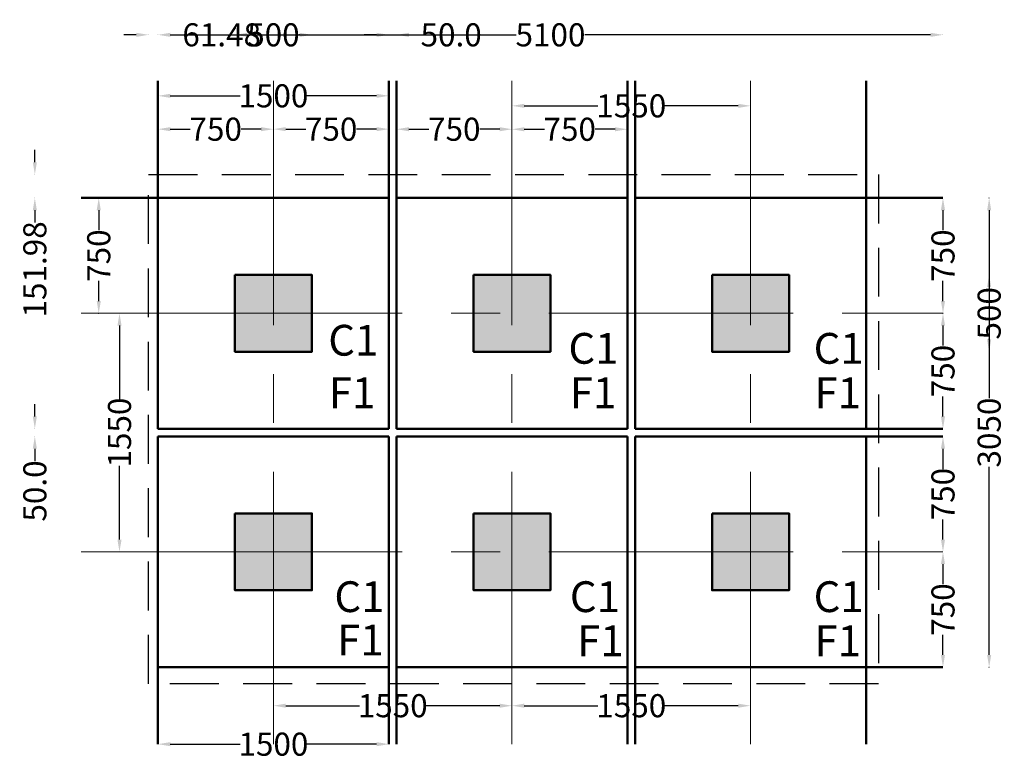
# Model space of a CAD drawing. Units: millimetres. Extents: x -19888 to 14444, y 67066 to 90098.
# Tile 4 of 7: x -19888 to -13491, y 82312 to 87118. Entities that reach past the tile are written whole.
import ezdxf

# ---------------------------------------------------------------- set-up
doc = ezdxf.new("R2010")
doc.units = ezdxf.units.MM
doc.header["$LTSCALE"] = 50
doc.header["$MEASUREMENT"] = 0
doc.linetypes.add('CENTER', pattern=[50.8, 31.75, -6.35, 6.35, -6.35])
doc.linetypes.add('HIDDEN', pattern=[9.525, 6.35, -3.175])
for name, color, linetype, lineweight in [('S-ANNO-DIMS', 2, 'Continuous', 18), ('S-ANNO-TEXT', 7, 'Continuous', 25), ('S-COLS', 4, 'Continuous', 50), ('S-FNDN', 1, 'Continuous', 50), ('S-FNDN-HIDN', 1, 'HIDDEN', 25), ('S-GRID', 8, 'CENTER', 18), ('S-PATT', 8, 'Continuous', 13)]:
    doc.layers.add(name, color=color, linetype=linetype, lineweight=lineweight)
doc.styles.get("Standard").update_dxf_attribs({"font": 'arial.ttf'})
doc.dimstyles.get("Standard").update_dxf_attribs({"dimtxt": 150, "dimasz": 80, "dimexe": 0.18, "dimexo": 0.0625, "dimgap": 0.09, "dimtad": 0, "dimdec": 0, "dimzin": 0, "dimdsep": 46, "dimtxsty": 'Standard', "dimcen": 0.09, "dimadec": 0, "dimazin": 0, "dimtfac": 1, "dimtdec": 0, "dimtofl": 0, "dimtmove": 0, "dimatfit": 3, "dimfxl": 1, "dimfxlon": 1, "dimtolj": 1, "dimtzin": 0, "dimarcsym": 0})

# ---------------------------------------------------------------- blocks, each defined once
blk = doc.blocks.new('*D1')
at = {"layer": 'Defpoints', "color": 0, "transparency": 16777216}
for p in [(-18989.3, 86406.7), (-18239.3, 86406.7), (-18239.3, 86406.7)]:
    blk.add_point(p, dxfattribs=at)
at = {"layer": 'S-ANNO-DIMS', "color": 0, "lineweight": -2, "transparency": 16777216}
for p, q in [((-18989.3, 86406.7), (-18989.3, 86406.9)), ((-18909.3, 86406.7), (-18779.2, 86406.7)), ((-18319.3, 86406.7), (-18449.3, 86406.7)), ((-18239.3, 86406.7), (-18239.3, 86406.9))]:
    blk.add_line(p, q, dxfattribs=at)
at = {"layer": 'S-ANNO-DIMS', "color": 0, "transparency": 16777216}
for points in [[(-18909.3, 86420.1), (-18909.3, 86393.4), (-18989.3, 86406.7)], [(-18319.3, 86420.1), (-18319.3, 86393.4), (-18239.3, 86406.7)]]:
    blk.add_solid(points, dxfattribs=at)
at = {"layer": 'S-ANNO-DIMS', "color": 0, "transparency": 16777216, "insert": (-18614.3, 86406.7), "char_height": 150, "attachment_point": 5}
blk.add_mtext('\\A1;750', dxfattribs=at)
blk = doc.blocks.new('*D2')
at = {"layer": 'Defpoints', "color": 0, "transparency": 16777216}
for p in [(-18239.3, 86406.7), (-17489.3, 86406.9), (-17489.3, 86406.7)]:
    blk.add_point(p, dxfattribs=at)
at = {"layer": 'S-ANNO-DIMS', "color": 0, "lineweight": -2, "transparency": 16777216}
for p, q in [((-18239.3, 86406.8), (-18239.3, 86407.1)), ((-18159.3, 86406.9), (-18029.2, 86406.9)), ((-17569.3, 86406.9), (-17699.3, 86406.9)), ((-17489.3, 86406.8), (-17489.3, 86407.1))]:
    blk.add_line(p, q, dxfattribs=at)
at = {"layer": 'S-ANNO-DIMS', "color": 0, "transparency": 16777216}
for points in [[(-18159.3, 86420.3), (-18159.3, 86393.6), (-18239.3, 86406.9)], [(-17569.3, 86420.3), (-17569.3, 86393.6), (-17489.3, 86406.9)]]:
    blk.add_solid(points, dxfattribs=at)
at = {"layer": 'S-ANNO-DIMS', "color": 0, "transparency": 16777216, "insert": (-17864.3, 86406.9), "char_height": 150, "attachment_point": 5}
blk.add_mtext('\\A1;750', dxfattribs=at)
blk = doc.blocks.new('*D3')
at = {"layer": 'Defpoints', "color": 0, "transparency": 16777216}
for p in [(-18989.3, 86719.9), (-17489.3, 86719.9), (-17489.3, 86623.5)]:
    blk.add_point(p, dxfattribs=at)
at = {"layer": 'S-ANNO-DIMS', "color": 0, "lineweight": -2, "transparency": 16777216}
for p, q in [((-18989.3, 86624.5), (-18989.3, 86623.3)), ((-18909.3, 86623.5), (-18456, 86623.5)), ((-17569.3, 86623.5), (-18022.5, 86623.5)), ((-17489.3, 86624.5), (-17489.3, 86623.3))]:
    blk.add_line(p, q, dxfattribs=at)
at = {"layer": 'S-ANNO-DIMS', "color": 0, "transparency": 16777216}
for points in [[(-18909.3, 86636.8), (-18909.3, 86610.2), (-18989.3, 86623.5)], [(-17569.3, 86636.8), (-17569.3, 86610.2), (-17489.3, 86623.5)]]:
    blk.add_solid(points, dxfattribs=at)
at = {"layer": 'S-ANNO-DIMS', "color": 0, "transparency": 16777216, "insert": (-18239.3, 86623.5), "char_height": 150, "attachment_point": 5}
blk.add_mtext('\\A1;1500', dxfattribs=at)
blk = doc.blocks.new('*D4')
at = {"layer": 'Defpoints', "color": 0, "transparency": 16777216}
for p in [(-17439.3, 86406.5), (-17439.3, 86406.5), (-16689.3, 86406.5)]:
    blk.add_point(p, dxfattribs=at)
at = {"layer": 'S-ANNO-DIMS', "color": 0, "lineweight": -2, "transparency": 16777216}
for p, q in [((-17439.3, 86406.5), (-17439.3, 86406.7)), ((-17359.3, 86406.5), (-17229.2, 86406.5)), ((-16769.3, 86406.5), (-16899.3, 86406.5)), ((-16689.3, 86406.5), (-16689.3, 86406.7))]:
    blk.add_line(p, q, dxfattribs=at)
at = {"layer": 'S-ANNO-DIMS', "color": 0, "transparency": 16777216}
for points in [[(-17359.3, 86419.8), (-17359.3, 86393.2), (-17439.3, 86406.5)], [(-16769.3, 86419.8), (-16769.3, 86393.2), (-16689.3, 86406.5)]]:
    blk.add_solid(points, dxfattribs=at)
at = {"layer": 'S-ANNO-DIMS', "color": 0, "transparency": 16777216, "insert": (-17064.3, 86406.5), "char_height": 150, "attachment_point": 5}
blk.add_mtext('\\A1;750', dxfattribs=at)
blk = doc.blocks.new('*D5')
at = {"layer": 'Defpoints', "color": 0, "transparency": 16777216}
for p in [(-16689.3, 86406.5), (-15939.3, 86406.5), (-15939.3, 86406.1)]:
    blk.add_point(p, dxfattribs=at)
at = {"layer": 'S-ANNO-DIMS', "color": 0, "lineweight": -2, "transparency": 16777216}
for p, q in [((-16689.3, 86406.4), (-16689.3, 86405.9)), ((-16609.3, 86406.1), (-16479.2, 86406.1)), ((-16019.3, 86406.1), (-16149.3, 86406.1)), ((-15939.3, 86406.4), (-15939.3, 86405.9))]:
    blk.add_line(p, q, dxfattribs=at)
at = {"layer": 'S-ANNO-DIMS', "color": 0, "transparency": 16777216}
for points in [[(-16609.3, 86419.5), (-16609.3, 86392.8), (-16689.3, 86406.1)], [(-16019.3, 86419.5), (-16019.3, 86392.8), (-15939.3, 86406.1)]]:
    blk.add_solid(points, dxfattribs=at)
at = {"layer": 'S-ANNO-DIMS', "color": 0, "transparency": 16777216, "insert": (-16314.3, 86406.1), "char_height": 150, "attachment_point": 5}
blk.add_mtext('\\A1;750', dxfattribs=at)
blk = doc.blocks.new('*D6')
at = {"layer": 'Defpoints', "color": 0, "transparency": 16777216}
for p in [(-16689.3, 86719.9), (-15139.3, 86719.9), (-16689.3, 86558.4)]:
    blk.add_point(p, dxfattribs=at)
at = {"layer": 'S-ANNO-DIMS', "color": 0, "lineweight": -2, "transparency": 16777216}
for p, q in [((-16689.3, 86559.4), (-16689.3, 86558.2)), ((-16609.3, 86558.4), (-16131, 86558.4)), ((-15219.3, 86558.4), (-15697.5, 86558.4)), ((-15139.3, 86559.4), (-15139.3, 86558.2))]:
    blk.add_line(p, q, dxfattribs=at)
at = {"layer": 'S-ANNO-DIMS', "color": 0, "transparency": 16777216}
for points in [[(-16609.3, 86571.7), (-16609.3, 86545.1), (-16689.3, 86558.4)], [(-15219.3, 86571.7), (-15219.3, 86545.1), (-15139.3, 86558.4)]]:
    blk.add_solid(points, dxfattribs=at)
at = {"layer": 'S-ANNO-DIMS', "color": 0, "transparency": 16777216, "insert": (-15914.3, 86558.4), "char_height": 150, "attachment_point": 5}
blk.add_mtext('\\A1;1550', dxfattribs=at)
blk = doc.blocks.new('*D7')
at = {"layer": 'Defpoints', "color": 0, "transparency": 16777216}
for p in [(-18989.3, 82410), (-17489.3, 82410), (-17489.3, 82410)]:
    blk.add_point(p, dxfattribs=at)
at = {"layer": 'S-ANNO-DIMS', "color": 0, "lineweight": -2, "transparency": 16777216}
for p, q in [((-18989.3, 82410), (-18989.3, 82410.2)), ((-18909.3, 82410), (-18456, 82410)), ((-17569.3, 82410), (-18022.5, 82410)), ((-17489.3, 82410), (-17489.3, 82410.2))]:
    blk.add_line(p, q, dxfattribs=at)
at = {"layer": 'S-ANNO-DIMS', "color": 0, "transparency": 16777216}
for points in [[(-18909.3, 82423.4), (-18909.3, 82396.7), (-18989.3, 82410)], [(-17569.3, 82423.4), (-17569.3, 82396.7), (-17489.3, 82410)]]:
    blk.add_solid(points, dxfattribs=at)
at = {"layer": 'S-ANNO-DIMS', "color": 0, "transparency": 16777216, "insert": (-18239.3, 82410), "char_height": 150, "attachment_point": 5}
blk.add_mtext('\\A1;1500', dxfattribs=at)
blk = doc.blocks.new('*D8')
at = {"layer": 'Defpoints', "color": 0, "transparency": 16777216}
for p in [(-18239.3, 82660), (-16689.3, 82660), (-16689.3, 82660)]:
    blk.add_point(p, dxfattribs=at)
at = {"layer": 'S-ANNO-DIMS', "color": 0, "lineweight": -2, "transparency": 16777216}
for p, q in [((-18239.3, 82660), (-18239.3, 82660.2)), ((-18159.3, 82660), (-17681, 82660)), ((-16769.3, 82660), (-17247.5, 82660)), ((-16689.3, 82660), (-16689.3, 82660.2))]:
    blk.add_line(p, q, dxfattribs=at)
at = {"layer": 'S-ANNO-DIMS', "color": 0, "transparency": 16777216}
for points in [[(-18159.3, 82673.4), (-18159.3, 82646.7), (-18239.3, 82660)], [(-16769.3, 82673.4), (-16769.3, 82646.7), (-16689.3, 82660)]]:
    blk.add_solid(points, dxfattribs=at)
at = {"layer": 'S-ANNO-DIMS', "color": 0, "transparency": 16777216, "insert": (-17464.3, 82660), "char_height": 150, "attachment_point": 5}
blk.add_mtext('\\A1;1550', dxfattribs=at)
blk = doc.blocks.new('*D9')
at = {"layer": 'Defpoints', "color": 0, "transparency": 16777216}
for p in [(-16689.3, 82653.4), (-15139.3, 82660), (-15139.3, 82660)]:
    blk.add_point(p, dxfattribs=at)
at = {"layer": 'S-ANNO-DIMS', "color": 0, "lineweight": -2, "transparency": 16777216}
for p, q in [((-16689.3, 82659), (-16689.3, 82660.2)), ((-16609.3, 82660), (-16131, 82660)), ((-15219.3, 82660), (-15697.5, 82660)), ((-15139.3, 82660), (-15139.3, 82660.2))]:
    blk.add_line(p, q, dxfattribs=at)
at = {"layer": 'S-ANNO-DIMS', "color": 0, "transparency": 16777216}
for points in [[(-16609.3, 82673.4), (-16609.3, 82646.7), (-16689.3, 82660)], [(-15219.3, 82673.4), (-15219.3, 82646.7), (-15139.3, 82660)]]:
    blk.add_solid(points, dxfattribs=at)
at = {"layer": 'S-ANNO-DIMS', "color": 0, "transparency": 16777216, "insert": (-15914.3, 82660), "char_height": 150, "attachment_point": 5}
blk.add_mtext('\\A1;1550', dxfattribs=at)
blk = doc.blocks.new('*D10')
at = {"layer": 'Defpoints', "color": 0, "ltscale": 50, "transparency": 16777216}
for p in [(-19239.3, 85210), (-19239.3, 83660), (-19239.3, 83660)]:
    blk.add_point(p, dxfattribs=at)
at = {"layer": 'S-ANNO-DIMS', "color": 0, "lineweight": -2, "ltscale": 50, "transparency": 16777216}
for p, q in [((-19239.3, 85210), (-19239.4, 85210)), ((-19239.3, 85130), (-19239.3, 84651.8)), ((-19239.3, 83740), (-19239.3, 84218.3)), ((-19239.3, 83660), (-19239.4, 83660))]:
    blk.add_line(p, q, dxfattribs=at)
at = {"layer": 'S-ANNO-DIMS', "color": 0, "ltscale": 50, "transparency": 16777216}
for points in [[(-19252.6, 85130), (-19225.9, 85130), (-19239.3, 85210)], [(-19252.6, 83740), (-19225.9, 83740), (-19239.3, 83660)]]:
    blk.add_solid(points, dxfattribs=at)
at = {"layer": 'S-ANNO-DIMS', "color": 0, "ltscale": 50, "transparency": 16777216, "insert": (-19239.3, 84435), "char_height": 150, "attachment_point": 5, "rotation": 90}
blk.add_mtext('\\A1;1550', dxfattribs=at)
blk = doc.blocks.new('*D11')
at = {"layer": 'Defpoints', "color": 0, "ltscale": 50, "transparency": 16777216}
for p in [(-19489.3, 85960), (-19374.1, 85960), (-19489.3, 85210)]:
    blk.add_point(p, dxfattribs=at)
at = {"layer": 'S-ANNO-DIMS', "color": 0, "lineweight": -2, "ltscale": 50, "transparency": 16777216}
for p, q in [((-19375.1, 85960), (-19373.9, 85960)), ((-19374.1, 85880), (-19374.1, 85750)), ((-19374.1, 85290), (-19374.1, 85420.1)), ((-19375.1, 85210), (-19373.9, 85210))]:
    blk.add_line(p, q, dxfattribs=at)
at = {"layer": 'S-ANNO-DIMS', "color": 0, "ltscale": 50, "transparency": 16777216}
for points in [[(-19387.4, 85880), (-19360.7, 85880), (-19374.1, 85960)], [(-19387.4, 85290), (-19360.7, 85290), (-19374.1, 85210)]]:
    blk.add_solid(points, dxfattribs=at)
at = {"layer": 'S-ANNO-DIMS', "color": 0, "ltscale": 50, "transparency": 16777216, "insert": (-19374.1, 85585), "char_height": 150, "attachment_point": 5, "rotation": 90}
blk.add_mtext('\\A1;750', dxfattribs=at)
blk = doc.blocks.new('*D12')
at = {"layer": 'Defpoints', "color": 0, "ltscale": 50, "transparency": 16777216}
for p in [(-13889.3, 85960), (-13889.3, 85210), (-13889.3, 85210)]:
    blk.add_point(p, dxfattribs=at)
at = {"layer": 'S-ANNO-DIMS', "color": 0, "lineweight": -2, "ltscale": 50, "transparency": 16777216}
for p, q in [((-13889.3, 85960), (-13889.4, 85960)), ((-13889.3, 85880), (-13889.3, 85750)), ((-13889.3, 85290), (-13889.3, 85420.1)), ((-13889.3, 85210), (-13889.4, 85210))]:
    blk.add_line(p, q, dxfattribs=at)
at = {"layer": 'S-ANNO-DIMS', "color": 0, "ltscale": 50, "transparency": 16777216}
for points in [[(-13902.6, 85880), (-13875.9, 85880), (-13889.3, 85960)], [(-13902.6, 85290), (-13875.9, 85290), (-13889.3, 85210)]]:
    blk.add_solid(points, dxfattribs=at)
at = {"layer": 'S-ANNO-DIMS', "color": 0, "ltscale": 50, "transparency": 16777216, "insert": (-13889.3, 85585), "char_height": 150, "attachment_point": 5, "rotation": 90}
blk.add_mtext('\\A1;750', dxfattribs=at)
blk = doc.blocks.new('*D13')
at = {"layer": 'Defpoints', "color": 0, "ltscale": 50, "transparency": 16777216}
for p in [(-13889.4, 85210.1), (-13889.3, 84460), (-13889.3, 84460)]:
    blk.add_point(p, dxfattribs=at)
at = {"layer": 'S-ANNO-DIMS', "color": 0, "lineweight": -2, "ltscale": 50, "transparency": 16777216}
for p, q in [((-13889.4, 85210.1), (-13889.1, 85210.1)), ((-13889.3, 85130.1), (-13889.3, 85000)), ((-13889.3, 84540), (-13889.3, 84670.1)), ((-13889.3, 84460), (-13889.4, 84460))]:
    blk.add_line(p, q, dxfattribs=at)
at = {"layer": 'S-ANNO-DIMS', "color": 0, "ltscale": 50, "transparency": 16777216}
for points in [[(-13902.6, 85130.1), (-13875.9, 85130.1), (-13889.3, 85210.1)], [(-13902.6, 84540), (-13875.9, 84540), (-13889.3, 84460)]]:
    blk.add_solid(points, dxfattribs=at)
at = {"layer": 'S-ANNO-DIMS', "color": 0, "ltscale": 50, "transparency": 16777216, "insert": (-13889.3, 84835), "char_height": 150, "attachment_point": 5, "rotation": 90}
blk.add_mtext('\\A1;750', dxfattribs=at)
blk = doc.blocks.new('*D14')
at = {"layer": 'Defpoints', "color": 0, "ltscale": 50, "transparency": 16777216}
for p in [(-13889.3, 84410), (-13889.3, 84410), (-13889.3, 83660)]:
    blk.add_point(p, dxfattribs=at)
at = {"layer": 'S-ANNO-DIMS', "color": 0, "lineweight": -2, "ltscale": 50, "transparency": 16777216}
for p, q in [((-13889.3, 84410), (-13889.4, 84410)), ((-13889.3, 84330), (-13889.3, 84200)), ((-13889.3, 83740), (-13889.3, 83870.1)), ((-13889.3, 83660), (-13889.4, 83660))]:
    blk.add_line(p, q, dxfattribs=at)
at = {"layer": 'S-ANNO-DIMS', "color": 0, "ltscale": 50, "transparency": 16777216}
for points in [[(-13902.6, 84330), (-13875.9, 84330), (-13889.3, 84410)], [(-13902.6, 83740), (-13875.9, 83740), (-13889.3, 83660)]]:
    blk.add_solid(points, dxfattribs=at)
at = {"layer": 'S-ANNO-DIMS', "color": 0, "ltscale": 50, "transparency": 16777216, "insert": (-13889.3, 84035), "char_height": 150, "attachment_point": 5, "rotation": 90}
blk.add_mtext('\\A1;750', dxfattribs=at)
blk = doc.blocks.new('*D15')
at = {"layer": 'Defpoints', "color": 0, "ltscale": 50, "transparency": 16777216}
for p in [(-13889.3, 83660), (-13889.3, 83660), (-13889.3, 82910)]:
    blk.add_point(p, dxfattribs=at)
at = {"layer": 'S-ANNO-DIMS', "color": 0, "lineweight": -2, "ltscale": 50, "transparency": 16777216}
for p, q in [((-13889.3, 83660), (-13889.4, 83660)), ((-13889.3, 83580), (-13889.3, 83450)), ((-13889.3, 82990), (-13889.3, 83120.1)), ((-13889.3, 82910), (-13889.4, 82910))]:
    blk.add_line(p, q, dxfattribs=at)
at = {"layer": 'S-ANNO-DIMS', "color": 0, "ltscale": 50, "transparency": 16777216}
for points in [[(-13902.6, 83580), (-13875.9, 83580), (-13889.3, 83660)], [(-13902.6, 82990), (-13875.9, 82990), (-13889.3, 82910)]]:
    blk.add_solid(points, dxfattribs=at)
at = {"layer": 'S-ANNO-DIMS', "color": 0, "ltscale": 50, "transparency": 16777216, "insert": (-13889.3, 83285), "char_height": 150, "attachment_point": 5, "rotation": 90}
blk.add_mtext('\\A1;750', dxfattribs=at)
blk = doc.blocks.new('*D24')
at = {"layer": 'Defpoints', "color": 0, "ltscale": 50, "transparency": 16777216}
for p in [(-17989.3, 87019.9), (-18489.3, 85460), (-17989.3, 85460)]:
    blk.add_point(p, dxfattribs=at)
at = {"layer": 'S-ANNO-DIMS', "color": 0, "lineweight": -2, "ltscale": 50, "transparency": 16777216}
for p, q in [((-18489.3, 87018.9), (-18489.3, 87020.1)), ((-18409.3, 87019.9), (-18404.8, 87019.9)), ((-18069.3, 87019.9), (-18073.7, 87019.9)), ((-17989.3, 87018.9), (-17989.3, 87020.1))]:
    blk.add_line(p, q, dxfattribs=at)
at = {"layer": 'S-ANNO-DIMS', "color": 0, "ltscale": 50, "transparency": 16777216}
for points in [[(-18409.3, 87033.2), (-18409.3, 87006.5), (-18489.3, 87019.9)], [(-18069.3, 87033.2), (-18069.3, 87006.5), (-17989.3, 87019.9)]]:
    blk.add_solid(points, dxfattribs=at)
at = {"layer": 'S-ANNO-DIMS', "color": 0, "ltscale": 50, "transparency": 16777216, "insert": (-18239.3, 87019.9), "char_height": 150, "attachment_point": 5}
blk.add_mtext('\\A1;500', dxfattribs=at)
blk = doc.blocks.new('*D25')
at = {"layer": 'Defpoints', "color": 0, "ltscale": 50, "transparency": 16777216}
for p in [(-17989.3, 85460), (-17989.3, 84960), (-13589.3, 84960)]:
    blk.add_point(p, dxfattribs=at)
at = {"layer": 'S-ANNO-DIMS', "color": 0, "lineweight": -2, "ltscale": 50, "transparency": 16777216}
for p, q in [((-13590.3, 85460), (-13589.1, 85460)), ((-13589.3, 85380), (-13589.3, 85375.6)), ((-13589.3, 85040), (-13589.3, 85044.5)), ((-13590.3, 84960), (-13589.1, 84960))]:
    blk.add_line(p, q, dxfattribs=at)
at = {"layer": 'S-ANNO-DIMS', "color": 0, "ltscale": 50, "transparency": 16777216}
for points in [[(-13602.6, 85380), (-13575.9, 85380), (-13589.3, 85460)], [(-13602.6, 85040), (-13575.9, 85040), (-13589.3, 84960)]]:
    blk.add_solid(points, dxfattribs=at)
at = {"layer": 'S-ANNO-DIMS', "color": 0, "ltscale": 50, "transparency": 16777216, "insert": (-13589.3, 85210), "char_height": 150, "attachment_point": 5, "rotation": 90}
blk.add_mtext('\\A1;500', dxfattribs=at)
blk = doc.blocks.new('*D26')
at = {"layer": 'Defpoints', "color": 0, "ltscale": 50, "transparency": 16777216}
for p in [(-13889.3, 87019.9), (-18989.3, 85960), (-13889.3, 85960)]:
    blk.add_point(p, dxfattribs=at)
at = {"layer": 'S-ANNO-DIMS', "color": 0, "lineweight": -2, "ltscale": 50, "transparency": 16777216}
for p, q in [((-18989.3, 87018.9), (-18989.3, 87020.1)), ((-18909.3, 87019.9), (-16663.1, 87019.9)), ((-13969.3, 87019.9), (-16215.5, 87019.9)), ((-13889.3, 87018.9), (-13889.3, 87020.1))]:
    blk.add_line(p, q, dxfattribs=at)
at = {"layer": 'S-ANNO-DIMS', "color": 0, "ltscale": 50, "transparency": 16777216}
for points in [[(-18909.3, 87033.2), (-18909.3, 87006.5), (-18989.3, 87019.9)], [(-13969.3, 87033.2), (-13969.3, 87006.5), (-13889.3, 87019.9)]]:
    blk.add_solid(points, dxfattribs=at)
at = {"layer": 'S-ANNO-DIMS', "color": 0, "ltscale": 50, "transparency": 16777216, "insert": (-16439.3, 87019.9), "char_height": 150, "attachment_point": 5}
blk.add_mtext('\\A1;5100', dxfattribs=at)
blk = doc.blocks.new('*D27')
at = {"layer": 'Defpoints', "color": 0, "ltscale": 50, "transparency": 16777216}
for p in [(-13889.3, 85960), (-13889.3, 82910), (-13589.3, 82910)]:
    blk.add_point(p, dxfattribs=at)
at = {"layer": 'S-ANNO-DIMS', "color": 0, "lineweight": -2, "ltscale": 50, "transparency": 16777216}
for p, q in [((-13590.3, 85960), (-13589.1, 85960)), ((-13589.3, 85880), (-13589.3, 84658.8)), ((-13589.3, 82990), (-13589.3, 84211.3)), ((-13590.3, 82910), (-13589.1, 82910))]:
    blk.add_line(p, q, dxfattribs=at)
at = {"layer": 'S-ANNO-DIMS', "color": 0, "ltscale": 50, "transparency": 16777216}
for points in [[(-13602.6, 85880), (-13575.9, 85880), (-13589.3, 85960)], [(-13602.6, 82990), (-13575.9, 82990), (-13589.3, 82910)]]:
    blk.add_solid(points, dxfattribs=at)
at = {"layer": 'S-ANNO-DIMS', "color": 0, "ltscale": 50, "transparency": 16777216, "insert": (-13589.3, 84435), "char_height": 150, "attachment_point": 5, "rotation": 90}
blk.add_mtext('\\A1;3050', dxfattribs=at)
blk = doc.blocks.new('*D72')
at = {"layer": 'Defpoints', "color": 0, "ltscale": 50, "transparency": 16777216}
for p in [(-17439.3, 87019.9), (-17489.3, 85960), (-17439.3, 85960)]:
    blk.add_point(p, dxfattribs=at)
at = {"layer": 'S-ANNO-DIMS', "color": 0, "lineweight": -2, "ltscale": 50, "transparency": 16777216}
for p, q in [((-17569.3, 87019.9), (-17649.3, 87019.9)), ((-17489.3, 87018.9), (-17489.3, 87020.1)), ((-17439.3, 87018.9), (-17439.3, 87020.1)), ((-17359.3, 87019.9), (-17279.3, 87019.9))]:
    blk.add_line(p, q, dxfattribs=at)
at = {"layer": 'S-ANNO-DIMS', "color": 0, "ltscale": 50, "transparency": 16777216}
for points in [[(-17569.3, 87033.2), (-17569.3, 87006.5), (-17489.3, 87019.9)], [(-17359.3, 87033.2), (-17359.3, 87006.5), (-17439.3, 87019.9)]]:
    blk.add_solid(points, dxfattribs=at)
at = {"layer": 'S-ANNO-DIMS', "color": 0, "ltscale": 50, "transparency": 16777216, "insert": (-17084.6, 87019.9), "char_height": 150, "attachment_point": 5}
blk.add_mtext('\\A1;50.0', dxfattribs=at)
blk = doc.blocks.new('*D73')
at = {"layer": 'Defpoints', "color": 0, "ltscale": 50, "transparency": 16777216}
for p in [(-18989.3, 84460), (-19789.3, 84410), (-18989.3, 84410)]:
    blk.add_point(p, dxfattribs=at)
at = {"layer": 'S-ANNO-DIMS', "color": 0, "lineweight": -2, "ltscale": 50, "transparency": 16777216}
for p, q in [((-19789.3, 84540), (-19789.3, 84620)), ((-19788.3, 84460), (-19789.4, 84460)), ((-19788.3, 84410), (-19789.4, 84410)), ((-19789.3, 84330), (-19789.3, 84250))]:
    blk.add_line(p, q, dxfattribs=at)
at = {"layer": 'S-ANNO-DIMS', "color": 0, "ltscale": 50, "transparency": 16777216}
for points in [[(-19802.6, 84540), (-19775.9, 84540), (-19789.3, 84460)], [(-19802.6, 84330), (-19775.9, 84330), (-19789.3, 84410)]]:
    blk.add_solid(points, dxfattribs=at)
at = {"layer": 'S-ANNO-DIMS', "color": 0, "ltscale": 50, "transparency": 16777216, "insert": (-19789.3, 84055.4), "char_height": 150, "attachment_point": 5, "rotation": 90}
blk.add_mtext('\\A1;50.0', dxfattribs=at)
blk = doc.blocks.new('*D74')
at = {"layer": 'Defpoints', "color": 0, "ltscale": 50, "transparency": 16777216}
for p in [(-19050.8, 86112), (-19789.3, 85960), (-18989.3, 85960)]:
    blk.add_point(p, dxfattribs=at)
at = {"layer": 'S-ANNO-DIMS', "color": 0, "lineweight": -2, "ltscale": 50, "transparency": 16777216}
for p, q in [((-19789.3, 86192), (-19789.3, 86272)), ((-19788.3, 86112), (-19789.4, 86112)), ((-19788.3, 85960), (-19789.4, 85960)), ((-19789.3, 85880), (-19789.3, 85800))]:
    blk.add_line(p, q, dxfattribs=at)
at = {"layer": 'S-ANNO-DIMS', "color": 0, "ltscale": 50, "transparency": 16777216}
for points in [[(-19802.6, 86192), (-19775.9, 86192), (-19789.3, 86112)], [(-19802.6, 85880), (-19775.9, 85880), (-19789.3, 85960)]]:
    blk.add_solid(points, dxfattribs=at)
at = {"layer": 'S-ANNO-DIMS', "color": 0, "ltscale": 50, "transparency": 16777216, "insert": (-19789.3, 85495.5), "char_height": 150, "attachment_point": 5, "rotation": 90}
blk.add_mtext('\\A1;151.98', dxfattribs=at)
blk = doc.blocks.new('*D75')
at = {"layer": 'Defpoints', "color": 0, "ltscale": 50, "transparency": 16777216}
for p in [(-18989.3, 87019.9), (-19050.8, 86112), (-18989.3, 85960)]:
    blk.add_point(p, dxfattribs=at)
at = {"layer": 'S-ANNO-DIMS', "color": 0, "lineweight": -2, "ltscale": 50, "transparency": 16777216}
for p, q in [((-19130.8, 87019.9), (-19210.8, 87019.9)), ((-19050.8, 87018.9), (-19050.8, 87020.1)), ((-18989.3, 87018.9), (-18989.3, 87020.1)), ((-18909.3, 87019.9), (-18829.3, 87019.9))]:
    blk.add_line(p, q, dxfattribs=at)
at = {"layer": 'S-ANNO-DIMS', "color": 0, "ltscale": 50, "transparency": 16777216}
for points in [[(-19130.8, 87033.2), (-19130.8, 87006.5), (-19050.8, 87019.9)], [(-18909.3, 87033.2), (-18909.3, 87006.5), (-18989.3, 87019.9)]]:
    blk.add_solid(points, dxfattribs=at)
at = {"layer": 'S-ANNO-DIMS', "color": 0, "ltscale": 50, "transparency": 16777216, "insert": (-18575.5, 87019.9), "char_height": 150, "attachment_point": 5}
blk.add_mtext('\\A1;61.48', dxfattribs=at)

msp = doc.modelspace()

# ---------------------------------------------------------------- hatches: boundary and pattern name
at = {"layer": 'S-PATT'}
h = msp.add_hatch(dxfattribs=at)
h.set_pattern_fill('AR-SAND', color=256, scale=30)
h.set_pattern_definition([(37.5, (0, 0), (-1.8898, 57.804713), [0, -45.6, 0, -51, 0, -48.75]), (7.5, (0, 0), (53.0933, 84.66438), [0, -24.6, 0, -41.1, 0, -15.75]), (327.5, (-36.9, 0), (93.424256, 0.169772), [0, -15, 0, -54, 0, -70.5]), (317.5, (-36.9, 0), (90.1838, 26.33027), [0, -7.5, 0, -35.4, 0, -40.5])])
h.paths.add_polyline_path([(-18239.269, 85460.031), (-18489.269, 85460.031), (-18489.269, 85210.031), (-18239.269, 85210.031)])
h.paths.add_polyline_path([(-17989.269, 85460.031), (-18239.269, 85460.031), (-18239.269, 85210.031), (-17989.269, 85210.031)])
h.paths.add_polyline_path([(-17989.269, 85210.031), (-18239.269, 85210.031), (-18239.269, 84960.031), (-17989.269, 84960.031)])
h.paths.add_polyline_path([(-18239.269, 85210.031), (-18489.269, 85210.031), (-18489.269, 84960.031), (-18239.269, 84960.031)])
h.paths.add_polyline_path([(-16689.269, 85460.031), (-16939.269, 85460.031), (-16939.269, 85210.031), (-16689.269, 85210.031)])
h.paths.add_polyline_path([(-16439.269, 85460.031), (-16689.269, 85460.031), (-16689.269, 85210.031), (-16439.269, 85210.031)])
h.paths.add_polyline_path([(-16439.269, 85210.031), (-16689.269, 85210.031), (-16689.269, 84960.031), (-16439.269, 84960.031)])
h.paths.add_polyline_path([(-16689.269, 85210.031), (-16939.269, 85210.031), (-16939.269, 84960.031), (-16689.269, 84960.031)])
h.paths.add_polyline_path([(-15139.269, 85460.031), (-15389.269, 85460.031), (-15389.269, 85210.031), (-15139.269, 85210.031)])
h.paths.add_polyline_path([(-14889.269, 85460.031), (-15139.269, 85460.031), (-15139.269, 85210.031), (-14889.269, 85210.031)])
h.paths.add_polyline_path([(-14889.269, 85210.031), (-15139.269, 85210.031), (-15139.269, 84960.031), (-14889.269, 84960.031)])
h.paths.add_polyline_path([(-15139.269, 85210.031), (-15389.269, 85210.031), (-15389.269, 84960.031), (-15139.269, 84960.031)])
h.paths.add_polyline_path([(-15139.269, 83910.031), (-15389.269, 83910.031), (-15389.269, 83660.031), (-15139.269, 83660.031)])
h.paths.add_polyline_path([(-14889.269, 83910.031), (-15139.269, 83910.031), (-15139.269, 83660.031), (-14889.269, 83660.031)])
h.paths.add_polyline_path([(-14889.269, 83660.031), (-15139.269, 83660.031), (-15139.269, 83410.031), (-14889.269, 83410.031)])
h.paths.add_polyline_path([(-15139.269, 83660.031), (-15389.269, 83660.031), (-15389.269, 83410.031), (-15139.269, 83410.031)])
h.paths.add_polyline_path([(-16439.269, 83910.031), (-16689.269, 83910.031), (-16689.269, 83660.031), (-16439.269, 83660.031)])
h.paths.add_polyline_path([(-16439.269, 83660.031), (-16689.269, 83660.031), (-16689.269, 83410.031), (-16439.269, 83410.031)])
h.paths.add_polyline_path([(-16689.269, 83660.031), (-16939.269, 83660.031), (-16939.269, 83410.031), (-16689.269, 83410.031)])
h.paths.add_polyline_path([(-16689.269, 83910.031), (-16939.269, 83910.031), (-16939.269, 83660.031), (-16689.269, 83660.031)])
h.paths.add_polyline_path([(-17989.269, 83910.031), (-18239.269, 83910.031), (-18239.269, 83660.031), (-17989.269, 83660.031)])
h.paths.add_polyline_path([(-18239.269, 83910.031), (-18489.269, 83910.031), (-18489.269, 83660.031), (-18239.269, 83660.031)])
h.paths.add_polyline_path([(-18239.269, 83660.031), (-18489.269, 83660.031), (-18489.269, 83410.031), (-18239.269, 83410.031)])
h.paths.add_polyline_path([(-17989.269, 83660.031), (-18239.269, 83660.031), (-18239.269, 83410.031), (-17989.269, 83410.031)])

# ---------------------------------------------------------------- linework, layer by layer
at = {"layer": 'S-COLS'}
for points in [[(-18489.269, 85460.031), (-17989.269, 85460.031), (-17989.269, 84960.031), (-18489.269, 84960.031)], [(-16939.269, 85460.031), (-16439.269, 85460.031), (-16439.269, 84960.031), (-16939.269, 84960.031)], [(-15389.269, 85460.031), (-14889.269, 85460.031), (-14889.269, 84960.031), (-15389.269, 84960.031)], [(-18489.269, 83910.031), (-17989.269, 83910.031), (-17989.269, 83410.031), (-18489.269, 83410.031)], [(-16939.269, 83910.031), (-16439.269, 83910.031), (-16439.269, 83410.031), (-16939.269, 83410.031)], [(-15389.269, 83910.031), (-14889.269, 83910.031), (-14889.269, 83410.031), (-15389.269, 83410.031)]]:
    msp.add_lwpolyline(points, close=True, dxfattribs=at)
at = {"layer": 'S-FNDN'}
for p, q in [((-18989.269, 86719.871), (-18989.269, 84460.031)), ((-17489.269, 86719.871), (-17489.269, 84460.031)), ((-17439.269, 86719.871), (-17439.269, 84460.031)), ((-15939.269, 86719.871), (-15939.269, 84460.031)), ((-15889.269, 86719.871), (-15889.269, 84460.031)), ((-14389.269, 86719.871), (-14389.269, 84460.031)), ((-18989.269, 85960.031), (-17489.269, 85960.031)), ((-17439.269, 85960.031), (-15939.269, 85960.031)), ((-15889.269, 85960.031), (-14389.269, 85960.031)), ((-18989.269, 84460.031), (-17489.269, 84460.031)), ((-17439.269, 84460.031), (-15939.269, 84460.031)), ((-15889.269, 84460.031), (-14389.269, 84460.031)), ((-18989.269, 84410.031), (-17489.269, 84410.031)), ((-18989.269, 84410.031), (-18989.269, 82910.031)), ((-17489.269, 84410.031), (-17489.269, 82910.031)), ((-17439.269, 84410.031), (-15939.269, 84410.031)), ((-17439.269, 84410.031), (-17439.269, 82910.031)), ((-15939.269, 84410.031), (-15939.269, 82910.031)), ((-15889.269, 84410.031), (-14389.269, 84410.031)), ((-15889.269, 84410.031), (-15889.269, 82910.031)), ((-14389.269, 84410.031), (-14389.269, 82910.031)), ((-18989.269, 82910.031), (-17489.269, 82910.031)), ((-18989.269, 82910.031), (-18989.269, 82860.031)), ((-17489.269, 82910.031), (-17489.269, 82410.031)), ((-17439.269, 82910.031), (-15939.269, 82910.031)), ((-17439.269, 82910.031), (-17439.269, 82410.031)), ((-15939.269, 82910.031), (-15939.269, 82410.031)), ((-15889.269, 82910.031), (-14389.269, 82910.031)), ((-15889.269, 82910.031), (-15889.269, 82410.031)), ((-14389.269, 82910.031), (-14389.269, 82410.031)), ((-18989.269, 82860.031), (-18989.269, 82410.031))]:
    msp.add_line(p, q, dxfattribs=at)
at = {"layer": 'S-FNDN', "ltscale": 50}
for p, q in [((-18989.269, 85960.031), (-19489.269, 85960.031)), ((-14389.269, 85960.031), (-13889.269, 85960.031)), ((-14389.269, 84460.031), (-13889.269, 84460.031)), ((-14389.269, 84410.031), (-13889.269, 84410.031)), ((-14389.269, 82910.031), (-13889.269, 82910.031))]:
    msp.add_line(p, q, dxfattribs=at)
at = {"layer": 'S-FNDN-HIDN'}
msp.add_lwpolyline([(-19050.751, 86112.01), (-14308.069, 86112.01), (-14308.069, 82803.153), (-19050.751, 82803.153)], close=True, dxfattribs=at)
at = {"layer": 'S-GRID'}
for p, q in [((-18239.269, 86719.871), (-18239.269, 82910.031)), ((-16689.269, 86719.871), (-16689.269, 82910.031)), ((-15139.269, 86719.871), (-15139.269, 82910.031)), ((-18989.269, 85210.031), (-14389.269, 85210.031)), ((-18989.269, 83660.031), (-14389.269, 83660.031)), ((-18239.269, 82910.031), (-18239.269, 82410.031)), ((-16689.269, 82910.031), (-16689.269, 82410.031)), ((-15139.269, 82910.031), (-15139.269, 82410.031))]:
    msp.add_line(p, q, dxfattribs=at)
at = {"layer": 'S-GRID', "ltscale": 50}
for p, q in [((-18989.269, 85210.031), (-19489.269, 85210.031)), ((-14389.269, 85210.031), (-13889.269, 85210.031)), ((-18989.269, 83660.031), (-19489.269, 83660.031)), ((-14389.269, 83660.031), (-13889.269, 83660.031))]:
    msp.add_line(p, q, dxfattribs=at)

# ---------------------------------------------------------------- texts
at = {"layer": 'S-ANNO-TEXT', "ltscale": 50, "char_height": 200, "attachment_point": 1}
for s, insert in [('C1', (-17882.957, 85135.079)), ('C1', (-16322.828, 85082.328)), ('C1', (-14729.746, 85082.328)), ('F1', (-17879.237, 84793.229)), ('F1', (-16313.42, 84793.229)), ('F1', (-14724.043, 84793.229)), ('C1', (-17843.27, 83468.477)), ('C1', (-16313.42, 83468.477)), ('C1', (-14729.746, 83468.477)), ('F1', (-17825.655, 83186.672)), ('F1', (-16266.042, 83181.787)), ('F1', (-14724.043, 83181.787))]:
    msp.add_mtext_dynamic_manual_height_columns(s, width=1609.35955, gutter_width=1, heights=[0], dxfattribs=dict(at, insert=insert))

# ---------------------------------------------------------------- dimensions: what is measured, and where the dimension line sits
at = {"layer": 'S-ANNO-DIMS', "ltscale": 50}
for base, p1, p2, override, picture, middle in [((-18989.269, 87019.871), (-19050.751, 86112.01), (-18989.269, 85960.031), {"dimdec": 2, "dimlfac": 1, "dimrnd": 0, "dimzin": 0, "dimdsep": 46, "dimlunit": 2}, '*D75', (-18575.529, 87019.871)), ((-13889.269, 87019.871), (-18989.269, 85960.031), (-13889.269, 85960.031), {"dimdec": 0, "dimlfac": 1, "dimrnd": 0, "dimzin": 0, "dimdsep": 46, "dimlunit": 2}, '*D26', (-16439.269, 87019.871)), ((-17989.269, 87019.871), (-18489.269, 85460.031), (-17989.269, 85460.031), {"dimdec": 0, "dimlfac": 1, "dimrnd": 0, "dimzin": 0, "dimdsep": 46, "dimlunit": 2}, '*D24', (-18239.269, 87019.871)), ((-17439.269, 87019.871), (-17489.269, 85960.031), (-17439.269, 85960.031), {"dimdec": 1, "dimlfac": 1, "dimrnd": 0, "dimzin": 0, "dimdsep": 46, "dimlunit": 2}, '*D72', (-17084.619, 87019.871))]:
    dim = msp.add_linear_dim(base=base, p1=p1, p2=p2, dimstyle='Standard', override=override, dxfattribs=at)
    dim.commit()
    dim.dimension.update_dxf_attribs({"geometry": picture, "text_midpoint": middle})
at = {"layer": 'S-ANNO-DIMS'}
for base, p1, p2, picture, middle in [((-17489.269, 86623.485), (-18989.269, 86719.871), (-17489.269, 86719.871), '*D3', (-18239.269, 86623.485)), ((-16689.269, 86558.39), (-15139.269, 86719.871), (-16689.269, 86719.871), '*D6', (-15914.269, 86558.39)), ((-18239.269, 86406.737), (-18989.269, 86406.737), (-18239.269, 86406.737), '*D1', (-18614.269, 86406.737)), ((-17489.269, 86406.917), (-18239.269, 86406.737), (-17489.269, 86406.737), '*D2', (-17864.269, 86406.917)), ((-17439.269, 86406.502), (-16689.269, 86406.502), (-17439.269, 86406.502), '*D4', (-17064.269, 86406.502)), ((-15939.269, 86406.122), (-16689.269, 86406.502), (-15939.269, 86406.502), '*D5', (-16314.269, 86406.122)), ((-16689.269, 82660.031), (-18239.269, 82660.031), (-16689.269, 82660.031), '*D8', (-17464.269, 82660.031)), ((-15139.269, 82660.031), (-16689.269, 82653.364), (-15139.269, 82660.031), '*D9', (-15914.269, 82660.031)), ((-17489.269, 82410.031), (-18989.269, 82410.031), (-17489.269, 82410.031), '*D7', (-18239.269, 82410.031))]:
    dim = msp.add_linear_dim(base=base, p1=p1, p2=p2, dimstyle='Standard', override={"dimclrd": 0, "dimclre": 0, "dimclrt": 0}, dxfattribs=at)
    dim.commit()
    dim.dimension.update_dxf_attribs({"geometry": picture, "text_midpoint": middle})
at = {"layer": 'S-ANNO-DIMS', "ltscale": 50}
for base, p1, p2, override, picture, middle in [((-19789.269, 85960.031), (-19050.751, 86112.01), (-18989.269, 85960.031), {"dimdec": 2, "dimlfac": 1, "dimrnd": 0, "dimzin": 0, "dimdsep": 46, "dimlunit": 2}, '*D74', (-19789.269, 85495.49)), ((-19374.064, 85960.031), (-19489.269, 85210.031), (-19489.269, 85960.031), {"dimclrd": 0, "dimclre": 0, "dimclrt": 0}, '*D11', (-19374.064, 85585.031)), ((-13889.269, 85210.031), (-13889.269, 85960.031), (-13889.269, 85210.031), {"dimclrd": 0, "dimclre": 0, "dimclrt": 0}, '*D12', (-13889.269, 85585.031)), ((-13589.269, 82910.031), (-13889.269, 85960.031), (-13889.269, 82910.031), {"dimdec": 0, "dimlfac": 1, "dimrnd": 0, "dimzin": 0, "dimdsep": 46, "dimlunit": 2}, '*D27', (-13589.269, 84435.031)), ((-13589.269, 84960.031), (-17989.269, 85460.031), (-17989.269, 84960.031), {"dimdec": 0, "dimlfac": 1, "dimrnd": 0, "dimzin": 0, "dimdsep": 46, "dimlunit": 2}, '*D25', (-13589.269, 85210.031)), ((-19239.269, 83660.031), (-19239.269, 85210.031), (-19239.269, 83660.031), {"dimclrd": 0, "dimclre": 0, "dimclrt": 0}, '*D10', (-19239.269, 84435.031)), ((-13889.269, 84460.031), (-13889.444, 85210.06), (-13889.269, 84460.031), {"dimclrd": 0, "dimclre": 0, "dimclrt": 0}, '*D13', (-13889.269, 84835.046)), ((-19789.269, 84410.031), (-18989.269, 84460.031), (-18989.269, 84410.031), {"dimdec": 1, "dimlfac": 1, "dimrnd": 0, "dimzin": 0, "dimdsep": 46, "dimlunit": 2}, '*D73', (-19789.269, 84055.381)), ((-13889.269, 84410.031), (-13889.269, 83660.031), (-13889.269, 84410.031), {"dimclrd": 0, "dimclre": 0, "dimclrt": 0}, '*D14', (-13889.269, 84035.031)), ((-13889.269, 83660.031), (-13889.269, 82910.031), (-13889.269, 83660.031), {"dimclrd": 0, "dimclre": 0, "dimclrt": 0}, '*D15', (-13889.269, 83285.031))]:
    dim = msp.add_linear_dim(base=base, p1=p1, p2=p2, angle=90, dimstyle='Standard', override=override, dxfattribs=at)
    dim.commit()
    dim.dimension.update_dxf_attribs({"geometry": picture, "text_midpoint": middle})

doc.saveas('drawing.dxf')
